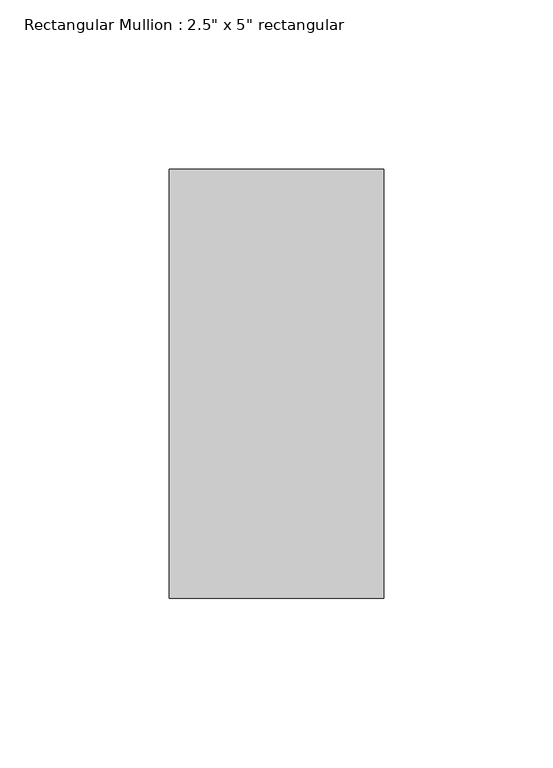
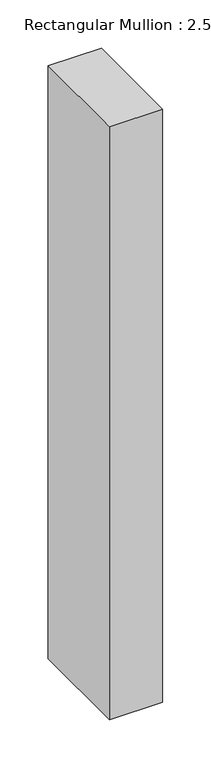
"""IFC4 building model written with IfcOpenShell, lengths in millimetres: member geometry."""

from ifc_helpers import new_model, si_unit, frame, origin, place, context, project, spatial, polyline, outline, extrude, source, transform, mapped, element, save


def member_c8dfd0df(model_context):
    return source(origin(), model_context, "Body", "SweptSolid", [
        extrude(outline(polyline([(0.0, 63.5), (0.0, -63.5), (-63.5, -63.5), (-63.5, 63.5), (0.0, 63.5)])), frame((0.0, 0.0, -748.4785678), z_axis=(0.0, 0.0, 1.0), x_axis=(1.0, 0.0, 0.0)), (0.0, 0.0, 1.0), 748.4785678),
    ])


if __name__ == "__main__":
    model = new_model("IFC4")
    model_context = context("Model", 3, world=origin())
    ifc_project = project(units=[si_unit("LENGTHUNIT", "METRE", prefix="MILLI")], contexts=[model_context])
    site = spatial("IfcSite", under=ifc_project)
    building = spatial("IfcBuilding", under=site)
    placement = place(None, origin())
    member_shape = member_c8dfd0df(model_context)
    element("IfcMember", 1, ObjectType="Rectangular Mullion : 2.5\" x 5\" rectangular", at=placement, inside=building, context=model_context, shape_type="MappedRepresentation", body=[
        mapped(member_shape, transform((0.0, 0.0, 0.0), x_axis=(1.0, 0.0, 0.0), y_axis=(0.0, 1.0, 0.0), z_axis=(0.0, 0.0, 1.0))),
    ])
    save(model, "model.ifc")

# Revit data of these elements
# Type "Rectangular Mullion : 2.5\" x 5\" rectangular"
#   built-in parameter 1007304 = 0.416667 (stored number, unit not read)
#   built-in parameter 1007301 = 0.104167 (stored number, unit not read)
#   built-in parameter 1007300 = 0.104167 (stored number, unit not read)
# Element 1 (IfcMember, "Rectangular Mullion : 2.5\" x 5\" rectangular")
#   Materials on its faces: "Aluminum"
# Materials
#   "Aluminum": class "Metal", colour RGB 247 247 247, transparency 0, Description = "Aluminum 6061", Cost = 0
